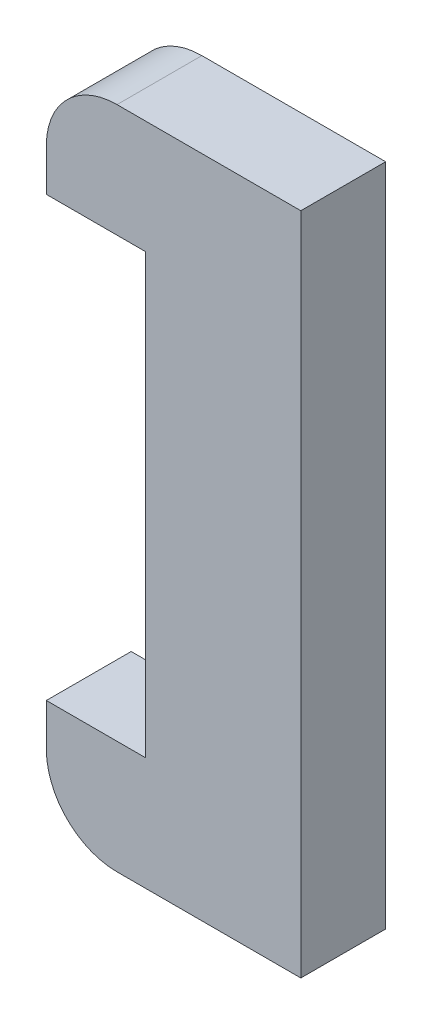
SolidWorks part; units mm, degrees
material "Plain Carbon Steel"
ref_plane "Front Plane" through (0, 0, 0) normal (0, 0, 1) x (1, 0, 0)
ref_plane "Top Plane" through (0, 0, 0) normal (0, 1, 0) x (1, 0, 0)
ref_plane "Right Plane" through (0, 0, 0) normal (1, 0, 0) x (0, 0, -1)
sketch "Gib Profile Sketch" plane through (0, 0, 0) normal (0, 0, 1) x (1, 0, 0)
  line L0 (-26, 30.1778) -> (0, 30.1778)
  line L1 (0, 30.1778) -> (0, -63.8222)
  line L2 (0, -63.8222) -> (-26, -63.8222)
  line L3 (-36, -53.8222) -> (-36, -47.8222)
  line L4 (-36, -47.8222) -> (-22, -47.8222)
  line L5 (-22, -47.8222) -> (-22, 14.1778)
  line L6 (-22, 14.1778) -> (-36, 14.1778)
  line L7 (-36, 14.1778) -> (-36, 20.1778)
  arc A0 (-26, -63.8222) -> (-36, -53.8222) centre (-26, -53.8222) cw
  arc A1 (-26, 30.1778) -> (-36, 20.1778) centre (-26, 20.1778) ccw
  point P11 (-36, -63.8222)
  point P14 (-36, 30.1778)
  dimension "D7" = 10
  dimension "D8" = 10
  dimension "D1" = 16
  dimension "D2" = 16
  dimension "D3" = 62
  dimension "D4" = 63.8222
  dimension "D5" = 22
  dimension "D6" = 14
extrude "Gib Body Extrude 12mm" add sketch "Gib Profile Sketch" along normal mid plane 12
